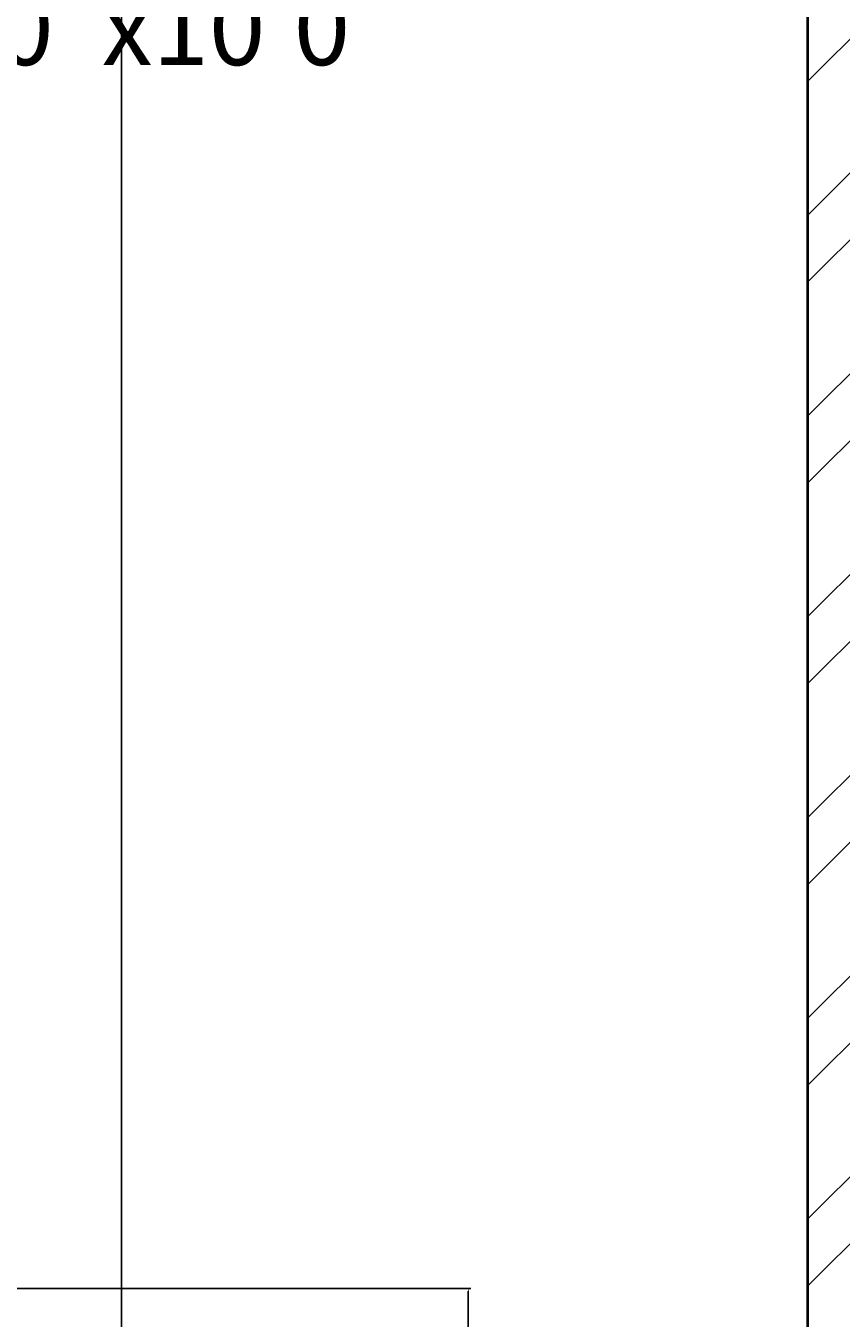
# Model space of a CAD drawing. Units: inches. Extents: x 2063 to 2617, y 1299 to 2210.
# Tile 12 of 22: x 2284 to 2338, y 1858 to 1945. Entities that reach past the tile are written whole.
import ezdxf

# ---------------------------------------------------------------- set-up
doc = ezdxf.new("R2010")
doc.units = ezdxf.units.IN
for name, color, linetype, lineweight in [('A-ANNO-DIMS', 2, 'Continuous', 18), ('A-AREA-IDEN', 7, 'Continuous', 18), ('A-WALL', 7, 'Continuous', 40)]:
    doc.layers.add(name, color=color, linetype=linetype, lineweight=lineweight)
doc.layers.add('A-WALL-PATT', color=215, linetype='Continuous', lineweight=13, true_color=0xa953a0)
doc.styles.get("Standard").update_dxf_attribs({"font": 'arial.ttf'})
doc.dimstyles.get("Standard").update_dxf_attribs({"dimtxt": 0.18, "dimasz": 0.18, "dimexe": 0.18, "dimexo": 0.0625, "dimgap": 0.09, "dimtad": 0, "dimtih": 1, "dimtoh": 1, "dimdec": 4, "dimzin": 0, "dimdsep": 46, "dimtxsty": 'Standard', "dimcen": 0.09, "dimadec": 0, "dimazin": 0, "dimtfac": 1, "dimtdec": 4, "dimtofl": 0, "dimtmove": 0, "dimatfit": 3, "dimfxl": 1, "dimtolj": 1, "dimtzin": 0, "dimarcsym": 0})

# ---------------------------------------------------------------- blocks, each defined once
blk = doc.blocks.new('*D59')
at = {"layer": 'A-ANNO-DIMS', "color": 0, "lineweight": -2, "transparency": 16777216}
for p, q in [((2290.144, 1554.562), (2290.144, 2170.742)), ((2290.324, 2170.562), (2315.07, 2170.562)), ((2340.464, 2170.562), (2315.719, 2170.562)), ((2340.644, 1554.562), (2340.644, 2170.742))]:
    blk.add_line(p, q, dxfattribs=at)
at = {"layer": 'A-ANNO-DIMS', "color": 0, "transparency": 16777216}
for points in [[(2290.324, 2170.592), (2290.324, 2170.532), (2290.144, 2170.562)], [(2340.464, 2170.592), (2340.464, 2170.532), (2340.644, 2170.562)]]:
    blk.add_solid(points, dxfattribs=at)
at = {"layer": 'Defpoints', "color": 0, "transparency": 16777216}
for p in [(2340.644, 2170.562), (2290.144, 1554.499), (2340.644, 1554.499)]:
    blk.add_point(p, dxfattribs=at)
at = {"layer": 'A-ANNO-DIMS', "color": 0, "transparency": 16777216, "insert": (2315.394, 2170.562), "char_height": 0.18, "attachment_point": 5}
blk.add_mtext('\\A1;50.5', dxfattribs=at)
blk = doc.blocks.new('*D69')
at = {"layer": 'A-ANNO-DIMS', "color": 0, "lineweight": -2, "transparency": 16777216}
for p, q in [((2271.707, 1860.051), (2313.574, 1860.051)), ((2313.394, 1859.871), (2313.394, 1845.204)), ((2313.394, 1830.174), (2313.394, 1844.84)), ((2271.707, 1829.994), (2313.574, 1829.994))]:
    blk.add_line(p, q, dxfattribs=at)
at = {"layer": 'A-ANNO-DIMS', "color": 0, "transparency": 16777216}
for points in [[(2313.364, 1859.871), (2313.424, 1859.871), (2313.394, 1860.051)], [(2313.364, 1830.174), (2313.424, 1830.174), (2313.394, 1829.994)]]:
    blk.add_solid(points, dxfattribs=at)
at = {"layer": 'Defpoints', "color": 0, "transparency": 16777216}
for p in [(2271.644, 1860.051), (2271.644, 1829.994), (2313.394, 1829.994)]:
    blk.add_point(p, dxfattribs=at)
at = {"layer": 'A-ANNO-DIMS', "color": 0, "transparency": 16777216, "insert": (2313.394, 1845.022), "char_height": 0.18, "attachment_point": 5}
blk.add_mtext('\\A1;30.057', dxfattribs=at)

msp = doc.modelspace()

# ---------------------------------------------------------------- hatches: boundary and pattern name
at = {"layer": 'A-WALL-PATT'}
h = msp.add_hatch(dxfattribs=at)
h.set_pattern_fill('ANSI32', color=256)
h.paths.add_polyline_path([(2553.6442, 2128.8122), (2511.1703, 2128.8122), (2511.1703, 2124.3122), (2549.1442, 2124.3122), (2549.1442, 2095.662), (2553.6442, 2095.662)])
h.paths.add_polyline_path([(2553.6442, 2035.662), (2549.1442, 2035.662), (2549.1442, 1980.3122), (2503.7214, 1980.3122), (2503.7214, 1975.8122), (2549.1442, 1975.8122), (2549.1442, 1962.9693), (2553.6442, 1962.9693)])
h.paths.add_polyline_path([(2553.6442, 1938.9693), (2549.1442, 1938.9693), (2549.1442, 1927.8122), (2477.1442, 1927.8122), (2477.1442, 1975.8122), (2481.2918, 1975.8122), (2481.2918, 1980.3122), (2453.2648, 1980.3122), (2453.2648, 1975.8122), (2472.6442, 1975.8122), (2472.6442, 1868.3122), (2400.6442, 1868.3122), (2400.6442, 1861.3782), (2405.1442, 1861.3782), (2405.1442, 1863.8122), (2480.9699, 1863.8122), (2480.9699, 1866.0622), (2480.9699, 1868.3122), (2477.1442, 1868.3122), (2477.1442, 1923.3122), (2549.1442, 1923.3122), (2549.1442, 1908.8504), (2553.6442, 1908.8504)])
h.paths.add_polyline_path([(2553.6442, 1884.8504), (2549.1442, 1884.8504), (2549.1442, 1868.3122), (2501.0636, 1868.3122), (2501.0636, 1863.8122), (2549.1442, 1863.8122), (2549.1442, 1826.0298), (2553.6442, 1826.0298)])
h.paths.add_polyline_path([(2388.1504, 1980.3122), (2340.6442, 1980.3122), (2340.6442, 2124.3122), (2358.7501, 2124.3122), (2358.7501, 2128.8122), (2316.3482, 2128.8122), (2316.3482, 2124.3122), (2336.1442, 2124.3122), (2336.1442, 1980.3122), (2289.1737, 1980.3122), (2289.1737, 1975.8122), (2336.1442, 1975.8122), (2336.1442, 1619.3122), (2333.1433, 1619.3122), (2333.1433, 1614.8122), (2344.1671, 1614.8122), (2344.1671, 1617.0622), (2344.1671, 1619.3122), (2340.6442, 1619.3122), (2340.6442, 1975.8122), (2388.1504, 1975.8122), (2388.1504, 1978.0622)])
h.paths.add_polyline_path([(2290.1442, 1614.8122), (2301.4594, 1614.8122), (2301.4594, 1617.0622), (2301.4594, 1619.3122), (2285.6442, 1619.3122), (2285.6442, 1566.8122), (2280.8619, 1566.8122), (2280.8619, 1564.5622), (2280.8619, 1562.3122), (2285.6442, 1562.3122), (2285.6442, 1442.3122), (2281.7879, 1442.3122), (2281.7879, 1437.8122), (2285.6442, 1437.8122), (2285.6442, 1401.8122), (2290.1442, 1401.8122)])
h.paths.add_polyline_path([(2549.1442, 1731.8122), (2405.1442, 1731.8122), (2405.1442, 1834.4638), (2402.8942, 1834.4638), (2400.6442, 1834.4638), (2400.6442, 1727.3122), (2549.1442, 1727.3122)])
h.paths.add_polyline_path([(2553.6442, 1766.0298), (2551.3942, 1766.0298), (2549.1442, 1766.0298), (2549.1442, 1686.7767), (2553.6442, 1686.7767)])
h.paths.add_polyline_path([(2553.6442, 1638.7767), (2551.3942, 1638.7767), (2549.1442, 1638.7767), (2549.1442, 1619.3122), (2448.6442, 1619.3122), (2448.6442, 1610.5671), (2450.8942, 1610.5671), (2453.1442, 1610.5671), (2453.1442, 1614.8122), (2549.1442, 1614.8122), (2549.1442, 1601.6421), (2553.6442, 1601.6421)])
h.paths.add_polyline_path([(2553.6442, 1577.6421), (2551.3942, 1577.6421), (2549.1442, 1577.6421), (2549.1442, 1566.8122), (2453.1442, 1566.8122), (2453.1442, 1591.5045), (2451.0335, 1591.5045), (2448.6442, 1591.5045), (2448.6442, 1566.8122), (2434.0475, 1566.8122), (2434.0475, 1562.3122), (2549.1442, 1562.3122), (2549.1442, 1533.48), (2553.6442, 1533.48)])
h.paths.add_polyline_path([(2553.6442, 1473.48), (2549.1442, 1473.48), (2549.1442, 1442.3122), (2502.6258, 1442.3122), (2502.6258, 1437.8122), (2549.1442, 1437.8122), (2549.1442, 1401.8122), (2553.6442, 1401.8122)])
h.paths.add_polyline_path([(2395.6442, 1562.3122), (2400.0901, 1562.3122), (2400.0901, 1564.5622), (2400.0901, 1566.8122), (2395.6442, 1566.8122), (2395.6442, 1619.3122), (2379.1127, 1619.3122), (2379.1127, 1614.8122), (2391.1442, 1614.8122), (2391.1442, 1401.8122), (2395.6442, 1401.8122), (2395.6442, 1437.8122), (2399.2425, 1437.8122), (2399.2425, 1440.0622), (2399.2425, 1442.3122), (2395.6442, 1442.3122)])
h.paths.add_polyline_path([(2442.6258, 1442.3122), (2419.6262, 1442.3122), (2419.6262, 1437.8122), (2442.6258, 1437.8122), (2442.6258, 1440.0622)])
h.paths.add_polyline_path([(2127.6442, 1480.2532), (2125.3942, 1480.2532), (2123.1442, 1480.2532), (2123.1442, 1401.8122), (2127.6442, 1401.8122), (2127.6442, 1437.8122), (2145.1538, 1437.8122), (2145.1538, 1440.0622), (2145.1538, 1442.3122), (2127.6442, 1442.3122)])
h.paths.add_polyline_path([(2259.809, 1442.3122), (2205.1538, 1442.3122), (2205.1538, 1437.8122), (2259.809, 1437.8122), (2259.809, 1440.0622)])
h.paths.add_polyline_path([(2127.6442, 1659.7652), (2123.1442, 1659.7652), (2123.1442, 1605.5161), (2125.3942, 1605.5161), (2127.6442, 1605.5161), (2127.6442, 1614.8122), (2223.6442, 1614.8122), (2223.6442, 1611.2723), (2228.1442, 1611.2723), (2228.1442, 1619.3122), (2127.6442, 1619.3122)])
h.paths.add_polyline_path([(2244.8673, 1566.8122), (2228.1442, 1566.8122), (2228.1442, 1590.8122), (2225.8942, 1590.8122), (2223.6442, 1590.8122), (2223.6442, 1566.8122), (2127.6442, 1566.8122), (2127.6442, 1581.5161), (2123.1442, 1581.5161), (2123.1442, 1540.2532), (2127.6442, 1540.2532), (2127.6442, 1562.3122), (2244.8673, 1562.3122), (2244.8673, 1564.5622)])
h.paths.add_polyline_path([(2172.5174, 1868.3122), (2127.6442, 1868.3122), (2127.6442, 1886.5833), (2123.1442, 1886.5833), (2123.1442, 1832.6633), (2127.6442, 1832.6633), (2127.6442, 1863.8122), (2172.5174, 1863.8122), (2172.5174, 1866.0622)])
h.paths.add_polyline_path([(2276.1442, 1868.3122), (2204.1442, 1868.3122), (2204.1442, 1923.3122), (2204.1442, 1975.8122), (2224.8362, 1975.8122), (2224.8362, 1978.1097), (2224.8362, 1980.3122), (2195.0729, 1980.3122), (2195.0729, 1978.0622), (2195.0729, 1975.8122), (2199.6442, 1975.8122), (2199.6442, 1927.8122), (2127.6442, 1927.8122), (2127.6442, 1942.3492), (2123.1442, 1942.3492), (2123.1442, 1910.5833), (2127.6442, 1910.5833), (2127.6442, 1923.3122), (2199.6442, 1923.3122), (2199.6442, 1868.3122), (2194.8228, 1868.3122), (2194.8228, 1864.7337), (2194.8228, 1863.8122), (2271.6442, 1863.8122), (2271.6442, 1860.0507), (2276.1442, 1860.0507)])
h.paths.add_polyline_path([(2276.1442, 1829.994), (2273.8942, 1829.994), (2271.6442, 1829.994), (2271.6442, 1731.8122), (2127.6442, 1731.8122), (2127.6442, 1772.6633), (2123.1442, 1772.6633), (2123.1442, 1707.7652), (2127.6442, 1707.7652), (2127.6442, 1727.3122), (2276.1442, 1727.3122)])
h.paths.add_polyline_path([(2127.6442, 2022.1152), (2123.1442, 2022.1152), (2123.1442, 1966.3492), (2127.6442, 1966.3492), (2127.6442, 1975.8122), (2174.2082, 1975.8122), (2174.2082, 1978.0622), (2174.2082, 1980.3122), (2127.6442, 1980.3122)])
h.paths.add_polyline_path([(2361.9755, 1678.588), (2398.4558, 1678.588), (2398.4558, 1697.2453), (2361.9755, 1697.2453)], flags=9)
h.paths.add_polyline_path([(2351.5397, 1780.4072), (2386.1987, 1780.4072), (2386.1987, 1790.7107), (2351.5397, 1790.7107)], flags=25)
h.paths.add_polyline_path([(2350.6753, 1940.9321), (2387.6024, 1940.9321), (2387.6024, 1959.5894), (2350.6753, 1959.5894)], flags=25)
h.paths.add_polyline_path([(2254.9545, 1684.638), (2295.0943, 1684.638), (2295.0943, 1703.2953), (2254.9545, 1703.2953)], flags=9)
h.paths.add_polyline_path([(2282.4946, 1782.4438), (2317.1535, 1782.4438), (2317.1535, 1792.7474), (2282.4946, 1792.7474)], flags=9)
h.paths.add_polyline_path([(2270.327, 1939.2854), (2307.254, 1939.2854), (2307.254, 1957.9428), (2270.327, 1957.9428)], flags=9)

# ---------------------------------------------------------------- linework, layer by layer
at = {"layer": 'A-WALL'}
msp.add_line((2336.1442, 1975.8122), (2336.1442, 1619.3122), dxfattribs=at)

# ---------------------------------------------------------------- texts
at = {"layer": 'A-AREA-IDEN', "insert": (2272.3376, 1955.4547), "char_height": 5, "attachment_point": 1}
msp.add_mtext_dynamic_manual_height_columns('DINING\\P11\'0"x10\'0"  ', width=126.60671, gutter_width=12.5, heights=[0], dxfattribs=at)

# ---------------------------------------------------------------- dimensions: what is measured, and where the dimension line sits
at = {"layer": 'A-ANNO-DIMS'}
dim = msp.add_linear_dim(base=(2340.6442, 2170.5622), p1=(2290.1442, 1554.4994), p2=(2340.6442, 1554.4994), dimstyle='Standard', override={"dimdec": 1, "dimlfac": 1, "dimrnd": 0, "dimzin": 0, "dimdsep": 46, "dimlunit": 2}, dxfattribs=at)
dim.commit()
dim.dimension.update_dxf_attribs({"geometry": '*D59', "text_midpoint": (2315.3942, 2170.5622)})
dim = msp.add_linear_dim(base=(2313.3943, 1829.994), p1=(2271.6442, 1860.0507), p2=(2271.6442, 1829.994), angle=270, dimstyle='Standard', override={"dimdec": 3, "dimlfac": 1, "dimrnd": 0, "dimzin": 0, "dimdsep": 46, "dimlunit": 2}, dxfattribs=at)
dim.commit()
dim.dimension.update_dxf_attribs({"geometry": '*D69', "text_midpoint": (2313.3943, 1845.0224)})

doc.saveas('drawing.dxf')
